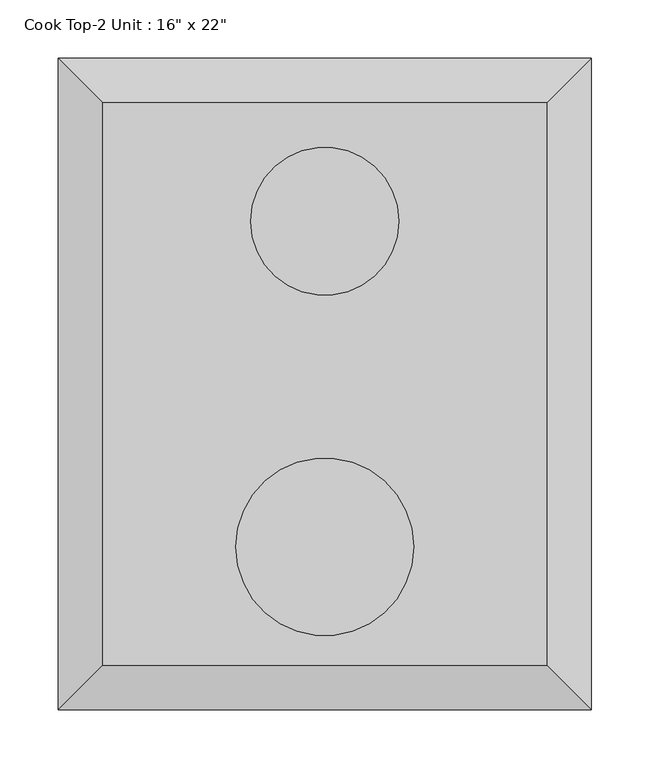
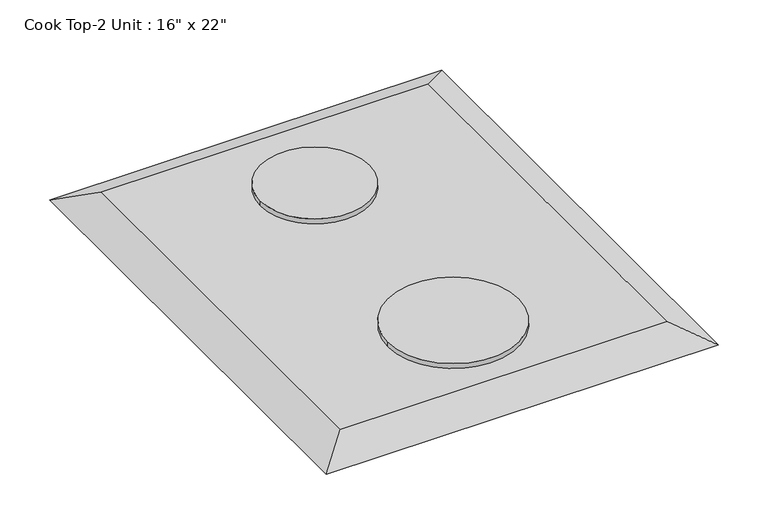
"""IFC4 building model written with IfcOpenShell, lengths in millimetres: proxy geometry."""

from ifc_helpers import new_model, si_unit, point, frame, frame_2d, origin, place, context, project, spatial, circle_curve, trimmed, segment, composite_curve, outline, extrude, faceted_brep, source, transform, mapped, element, save


def proxy_40295e01(model_context):
    return source(origin(), model_context, "Body", "SolidModel", [
        faceted_brep([(266.7, -271.5247956, 933.45), (266.7, 211.0752044, 933.45), (-114.3, 211.0752044, 933.45), (-114.3, -271.5247956, 933.45), (304.8, -309.6247956, 914.4), (-152.4, -309.6247956, 914.4), (-152.4, 249.1752044, 914.4), (304.8, 249.1752044, 914.4)], [[[0, 1, 2, 3]], [[4, 5, 6, 7]], [[4, 0, 3, 5]], [[5, 3, 2, 6]], [[6, 2, 1, 7]], [[7, 1, 0, 4]]]),
        extrude(outline(composite_curve([segment(trimmed(circle_curve(frame_2d((76.2, -169.9247956)), 76.2), [point((152.4, -169.9247956))], [point((0.0, -169.9247956))], False, "CARTESIAN"), True, "CONTINUOUS"), segment(trimmed(circle_curve(frame_2d((76.2, -169.9247956)), 76.2), [point((0.0, -169.9247956))], [point((152.4, -169.9247956))], False, "CARTESIAN"), True, "CONTINUOUS")], self_intersect=False)), frame((0.0, 0.0, 933.45), z_axis=(0.0, 0.0, 1.0), x_axis=(1.0, 0.0, 0.0)), (0.0, 0.0, 1.0), 6.35),
        extrude(outline(composite_curve([segment(trimmed(circle_curve(frame_2d((76.2, 109.4752044)), 63.5), [point((139.7, 109.4752044))], [point((12.7, 109.4752044))], False, "CARTESIAN"), True, "CONTINUOUS"), segment(trimmed(circle_curve(frame_2d((76.2, 109.4752044)), 63.5), [point((12.7, 109.4752044))], [point((139.7, 109.4752044))], False, "CARTESIAN"), True, "CONTINUOUS")], self_intersect=False)), frame((0.0, 0.0, 933.45), z_axis=(0.0, 0.0, 1.0), x_axis=(1.0, 0.0, 0.0)), (0.0, 0.0, 1.0), 6.35),
    ])


if __name__ == "__main__":
    model = new_model("IFC4")
    model_context = context("Model", 3, world=origin())
    ifc_project = project(units=[si_unit("LENGTHUNIT", "METRE", prefix="MILLI")], contexts=[model_context])
    site = spatial("IfcSite", under=ifc_project)
    building = spatial("IfcBuilding", under=site)
    placement = place(None, origin())
    proxy_shape = proxy_40295e01(model_context)
    element("IfcBuildingElementProxy", 1, Name="Cook Top-2 Unit : 16\" x 22\"", ObjectType="Cook Top-2 Unit : 16\" x 22\"", at=placement, inside=building, context=model_context, shape_type="MappedRepresentation", body=[
        mapped(proxy_shape, transform((0.0, 0.0, 0.0), x_axis=(1.0, 0.0, 0.0), y_axis=(0.0, 1.0, 0.0), z_axis=(0.0, 0.0, 1.0))),
    ])
    save(model, "model.ifc")

# Revit data of these elements
# Type "Cook Top-2 Unit : 16\" x 22\""
#   Assembly Code = "E1090400"
#   Counter Height = 3' - 0"
#   Depth = 1' - 10"
#   Width = 1' - 6"
#   Burner Material = Metal - Chrome
#   Cooktop Material = Metal - Steel, Polished
#   Default Elevation = 0
# Element 1 (IfcBuildingElementProxy, "Cook Top-2 Unit : 16\" x 22\"")
#   Materials on its faces: "Metal - Steel, Polished", "Metal - Chrome"
# Materials
#   "Metal - Chrome": colour RGB 57 57 57, transparency 0
#   "Metal - Steel, Polished": colour RGB 57 57 57, transparency 0
